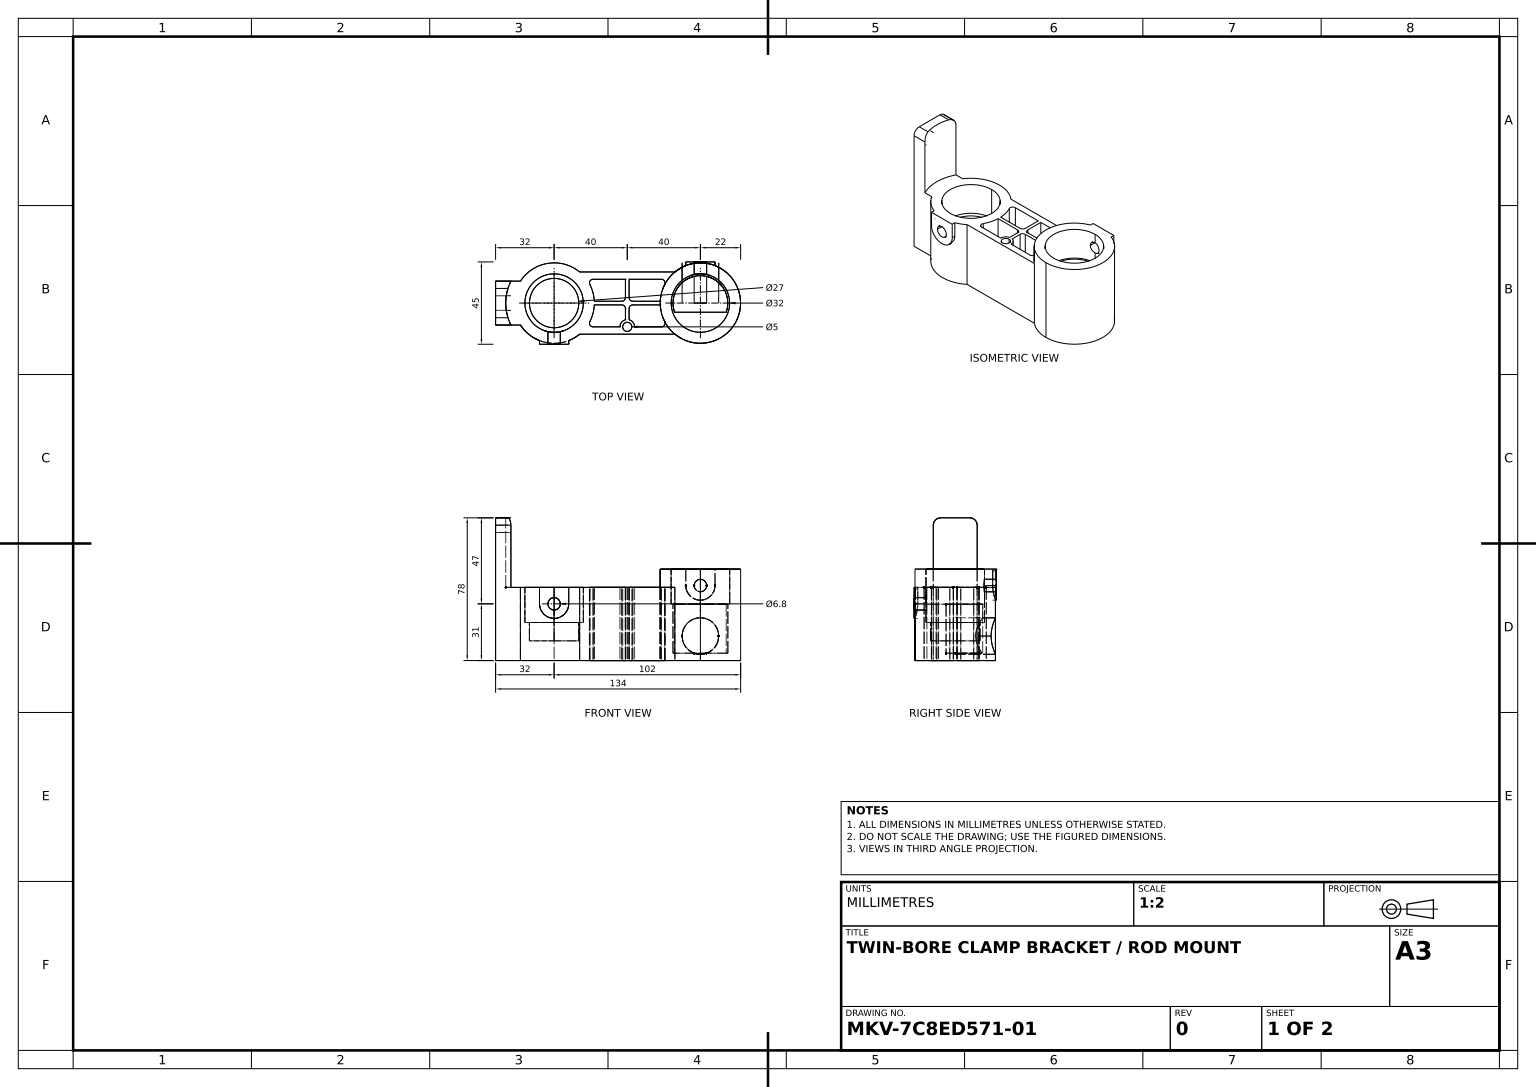
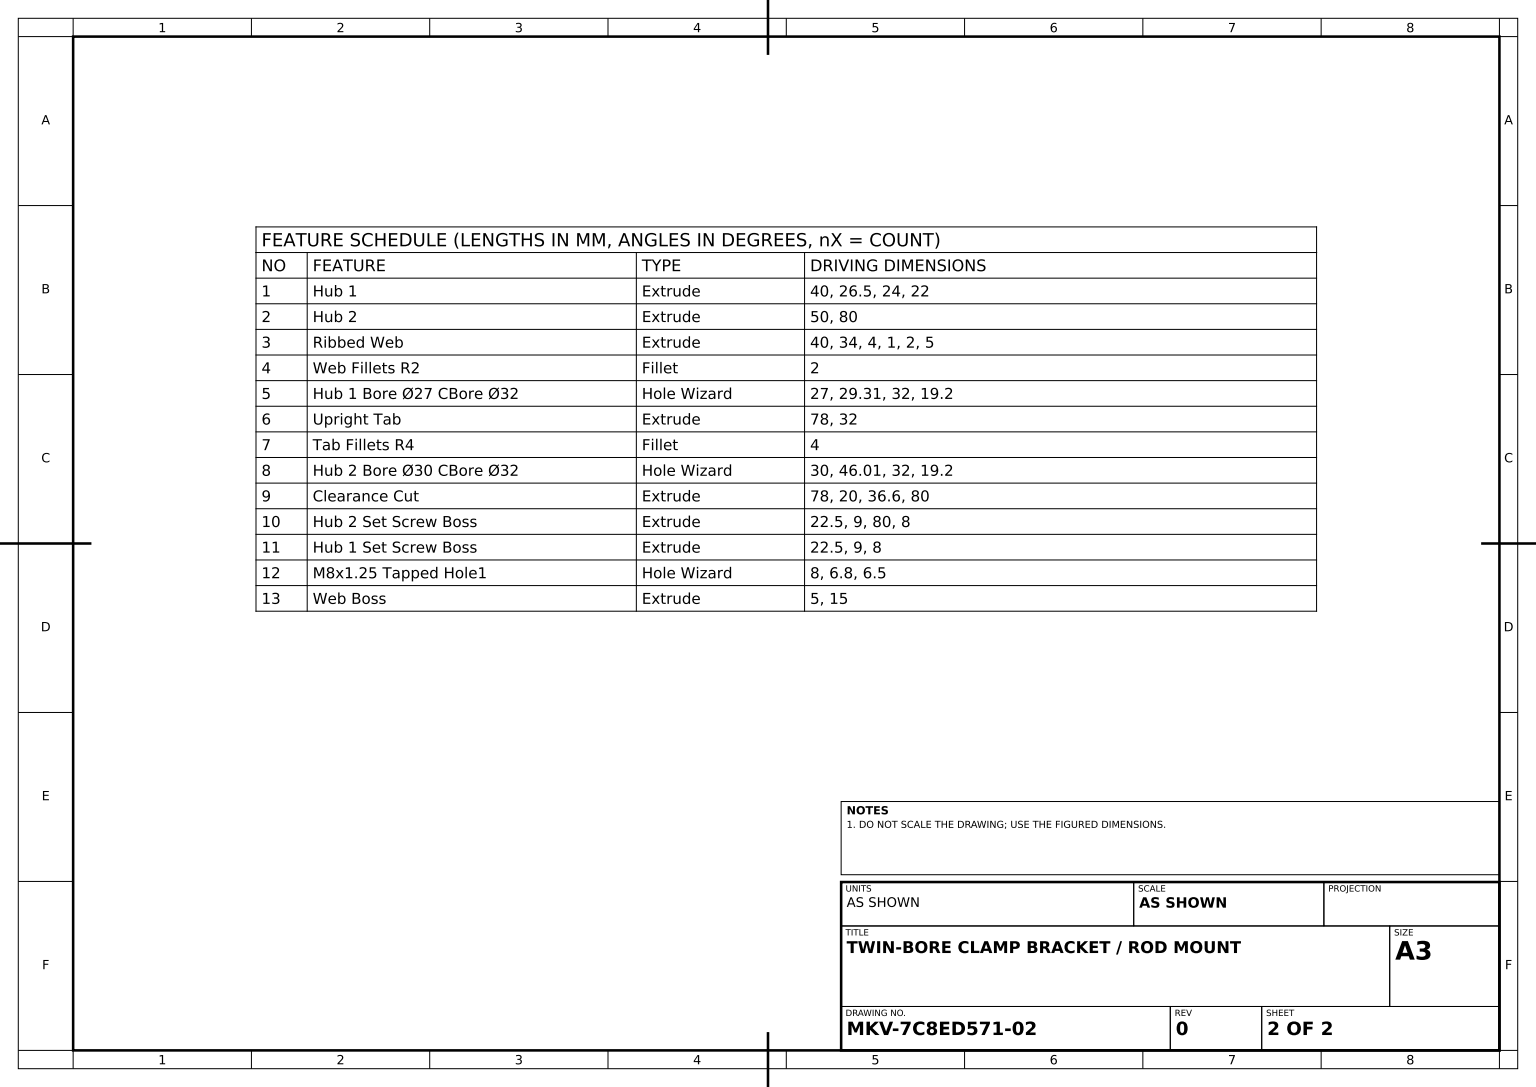
SolidWorks part; units mm, degrees
material "Plain Carbon Steel"
ref_plane "Front Plane" through (0, 0, 0) normal (0, 0, 1) x (1, 0, 0)
ref_plane "Top Plane" through (0, 0, 0) normal (0, 1, 0) x (1, 0, 0)
ref_plane "Right Plane" through (0, 0, 0) normal (1, 0, 0) x (0, 0, -1)
sketch "Hub 1 Sketch" plane through (0, 0, 0) normal (0, 1, 0) x (1, 0, 0)
  line L0 (0, 0) -> (-26.5, 0) construction
  line L1 (-23.6273, 12) -> (-18.4391, 12)
  line L2 (-23.6273, -12) -> (-18.4391, -12)
  arc A0 (-18.4391, -12) -> (-18.4391, 12) centre (0, 0) ccw
  arc A1 (-23.6273, 12) -> (-23.6273, -12) centre (0, 0) ccw
  dimension "D1" = 22
  dimension "D2" = 26.5
  dimension "D3" = 24
extrude "Hub 1" add sketch "Hub 1 Sketch" along normal blind 40
sketch "Hub 2 Sketch" plane through (0, 0, 0) normal (0, 1, 0) x (1, 0, 0)
  circle A0 centre (80, 0) radius 22
  arc A1 (-18.4391, -12) -> (-18.4391, 12) centre (0, 0) ccw construction
  dimension "D1" = 80
extrude "Hub 2" add sketch "Hub 2 Sketch" along normal blind 50 separate body
sketch "Ribbed Web Sketch" plane through (0, 0, 0) normal (0, 1, 0) x (1, 0, 0)
  line L0 (13.9642, 17) -> (66.0358, 17)
  line L1 (13.9642, -17) -> (66.0358, -17)
  line L2 (0, 0) -> (80, 0) construction
  line L3 (17.7482, 13) -> (39, 13)
  line L4 (17.7482, -13) -> (36, -13)
  line L5 (13.9642, 13) -> (66.0358, 13) construction
  line L6 (13.9642, -13) -> (66.0358, -13) construction
  line L7 (22, 0) -> (58, 0) construction
  line L8 (21.9773, -1) -> (39, -1)
  line L9 (21.9773, 1) -> (39, 1)
  line L10 (40, 1) -> (40, -9) construction
  line L11 (39, 13) -> (39, 1)
  line L12 (41, 13) -> (41, 1)
  line L13 (41, 17) -> (41, -17) construction
  line L14 (40, 17) -> (40, -17) construction
  line L15 (39, 17) -> (39, -17) construction
  line L16 (44, -13) -> (62.2518, -13)
  line L17 (41, 13) -> (62.2518, 13)
  line L18 (41, -1) -> (41, -9.127)
  line L19 (39, -1) -> (39, -9.127)
  line L20 (41, 1) -> (58.0227, 1)
  line L21 (22, 1) -> (58, 1) construction
  line L22 (41, -1) -> (58.0227, -1)
  line L23 (22, -1) -> (58, -1) construction
  line L24 (22, 0) -> (58, 0) construction
  arc A0 (-18.4391, -12) -> (-18.4391, 12) centre (0, 0) ccw construction
  circle A1 centre (80, 0) radius 22 construction
  arc A2 (66.0358, 17) -> (62.2518, 13) centre (80, 0) ccw
  arc A3 (13.9642, -17) -> (17.7482, -13) centre (0, 0) ccw
  arc A4 (62.2518, -13) -> (66.0358, -17) centre (80, 0) ccw
  arc A5 (17.7482, 13) -> (13.9642, 17) centre (0, 0) ccw
  arc A6 (13.9642, -17) -> (17.7482, -13) centre (0, 0) ccw
  arc A7 (17.7482, 13) -> (13.9642, 17) centre (0, 0) ccw
  arc A8 (13.9642, -17) -> (17.7482, -13) centre (0, 0) ccw
  arc A9 (17.7482, 13) -> (13.9642, 17) centre (0, 0) ccw
  arc A10 (21.9773, -1) -> (21.9773, 1) centre (0, 0) ccw
  arc A11 (58.0227, 1) -> (58.0227, -1) centre (80, 0) ccw
  arc A12 (62.2518, -13) -> (62.2518, 13) centre (80, 0) ccw
  arc A13 (44, -13) -> (41, -9.127) centre (40, -13) ccw
  arc A14 (39, -9.127) -> (36, -13) centre (40, -13) ccw
  circle A15 centre (40, -13) radius 2.5
  dimension "D9" = 4
  dimension "D10" = 5
  dimension "D1" = 34
  dimension "D8" = 40
  dimension "D6" = 2
  dimension "D7" = 1
  dimension "D2" = 4
  dimension "D3" = 4
  dimension "D4" = 1
  dimension "D5" = 1
extrude "Ribbed Web" add sketch "Ribbed Web Sketch" along normal blind 40 contours L19 A14 L4 A3 L1 A4 L16 A13 L18 L22 A11 L20 L12 L17 A2 L0 A5 L3 L11 L9 A10 L8 A15
fillet "Web Fillets R2" radius 2 8 edges at (62.2518, 20, 13) (62.2518, 20, -13) (17.7482, 20, -13) (17.7482, 20, 13) (39, 20, -1) (41, 20, -1) (41, 20, 1) (39, 20, 1)
hole_wizard "Hub 1 Bore Ø27 CBore Ø32" positions "3DSketch1" profile "Sketch4" legacy
sketch3d "3DSketch1"
  arc A0 (13.9642, 40, -17) -> (-18.4391, 40, -12) centre (0, 40, 0) ccw construction
  point P0 (0, 40, 0)
  point P6 (0, 62, 0)
sketch "Sketch4" plane through (0, 40, 0) normal (1, 0, 0) x (0, 0, 1)
  line L0 (0, 0) -> (0, 29.2032)
  line L1 (0, 29.2032) -> (13.5, 29.2032)
  line L2 (13.5, 29.2032) -> (13.5, 19.2)
  line L3 (13.5, 19.2) -> (16, 19.2)
  line L4 (16, 19.2) -> (16, 0)
  line L5 (16, 0) -> (0, 0)
  line L6 (0, 110) -> (0, -10) construction
  dimension "Diameter" = 27
  dimension "Depth" = 29.31
  dimension "C-Bore Diameter" = 32
  dimension "C-Bore Depth" = 19.2
sketch "Upright Tab Sketch" plane through (0, 0, 0) normal (0, 1, 0) x (1, 0, 0)
  line L0 (-23.6273, -12) -> (-18.4391, -12) construction
  line L1 (-23.6273, 12) -> (-32, 12)
  line L3 (-23.6273, -12) -> (-32, -12)
  line L4 (-32, 12) -> (-32, -12)
  arc A0 (-23.6273, 12) -> (-23.6273, -12) centre (0, 0) ccw construction
  arc A1 (-23.6273, 12) -> (-23.6273, -12) centre (0, 0) ccw
  dimension "D1" = 32
extrude "Upright Tab" add sketch "Upright Tab Sketch" along normal blind 78
fillet "Tab Fillets R4" radius 4 2 edges at (-27.8137, 78, -12) (-27.8137, 78, 12)
hole_wizard "Hub 2 Bore Ø30 CBore Ø32" positions "3DSketch2" profile "Sketch6" legacy
sketch3d "3DSketch2"
  circle A0 centre (80, 50, 0) radius 22 construction
  point P0 (80, 50, 0)
  point P5 (80, 72, 0)
sketch "Sketch6" plane through (80, 50, 0) normal (1, 0, 0) x (0, 0, 1)
  line L0 (0, 0) -> (0, 45.9991)
  line L1 (0, 45.9991) -> (15, 45.9991)
  line L2 (15, 45.9991) -> (15, 19.2)
  line L3 (15, 19.2) -> (16, 19.2)
  line L4 (16, 19.2) -> (16, 0)
  line L5 (16, 0) -> (0, 0)
  line L6 (0, 110) -> (0, -10) construction
  dimension "Diameter" = 30
  dimension "Depth" = 46.01
  dimension "C-Bore Diameter" = 32
  dimension "C-Bore Depth" = 19.2
sketch "Clearance Cut Sketch" plane through (0, 0, 0) normal (0, 0, 1) x (1, 0, 0)
  line L0 (102, 50) -> (58, 50) construction
  circle A0 centre (80, 13.4) radius 10
  dimension "D1" = 20
  dimension "D2" = 36.6
  dimension "D3" = 80
extrude "Clearance Cut" cut sketch "Clearance Cut Sketch" against normal blind 78
ref_plane "Hub 2 Set Screw Plane" through (0, 0, -22.5) normal (0, 0, 1) x (1, 0, 0)
sketch "Hub 2 Set Screw Boss Sketch" plane through (0, 0, -22.5) normal (0, 0, 1) x (1, 0, 0)
  line L0 (72, 41) -> (72, 50)
  line L1 (96, 50) -> (64, 50) construction
  line L2 (72, 50) -> (88, 50)
  line L3 (88, 50) -> (88, 41)
  arc A0 (72, 41) -> (88, 41) centre (80, 41) ccw
  dimension "D3" = 8
  dimension "D1" = 9
  dimension "D2" = 80
extrude "Hub 2 Set Screw Boss" add sketch "Hub 2 Set Screw Boss Sketch" along normal up to surface (2.0061 mm away)
ref_plane "Hub 1 Set Screw Plane" through (0, 0, 22.5) normal (0, 0, 1) x (1, 0, 0)
sketch "Hub 1 Set Screw Boss Sketch" plane through (0, 0, 22.5) normal (0, 0, 1) x (1, 0, 0)
  line L0 (-8, 31) -> (-8, 40)
  line L1 (13.9642, 40) -> (-18.4391, 40) construction
  line L2 (-8, 40) -> (8, 40)
  line L3 (8, 40) -> (8, 31)
  arc A0 (-8, 31) -> (8, 31) centre (0, 31) ccw
  dimension "D2" = 8
  dimension "D1" = 9
extrude "Hub 1 Set Screw Boss" add sketch "Hub 1 Set Screw Boss Sketch" against normal up to surface (2.0061 mm away)
hole_wizard "M8x1.25 Tapped Hole1" positions "3DSketch4" profile "Sketch13" tap size "M8x1.25" standard "ANSI Metric"
sketch3d "3DSketch4"
  arc A0 (-8, 31, 22.5) -> (8, 31, 22.5) centre (0, 31, 22.5) ccw construction
  arc A1 (72, 41, -22.5) -> (88, 41, -22.5) centre (80, 41, -22.5) ccw construction
  point P0 (80, 41, -22.5)
  point P2 (0, 31, 22.5)
  point P8 (0, 31, 30.5)
  point P12 (80, 41, -14.5)
sketch "Sketch13" plane through (80, 41, -22.5) normal (1, 0, 0) x (0, 1, 0)
  line L0 (0, 0) -> (0, 6.5)
  line L1 (0, 6.5) -> (3.4, 6.5)
  line L2 (3.4, 6.5) -> (3.4, 0)
  line L5 (3.4, 0) -> (0, 0)
  line L11 (0, -6.35) -> (0, 107.95) construction
  dimension "Thru Tap Drill Dia." = 6.8
  dimension "Thru Tap Drill Depth" = 6.5
cosmetic thread "Hole Thread1" parameters "D2"=8
cosmetic thread "Hole Thread2" parameters "D2"=8
sketch "Web Boss Sketch" plane through (0, 4.0009, 0) normal (0, 1, 0) x (1, 0, 0)
  line L0 (83.4141, 0) -> (76.5859, 0) construction
  line L1 (65.8579, -5) -> (94.1421, -5)
  arc A0 (65.8579, -5) -> (94.1421, -5) centre (80, 0) ccw
  dimension "D2" = 15
  dimension "D1" = 5
extrude "Web Boss" add sketch "Web Boss Sketch" along normal up to surface (26.7991 mm away) up to face at (80, 30.8, 15)
